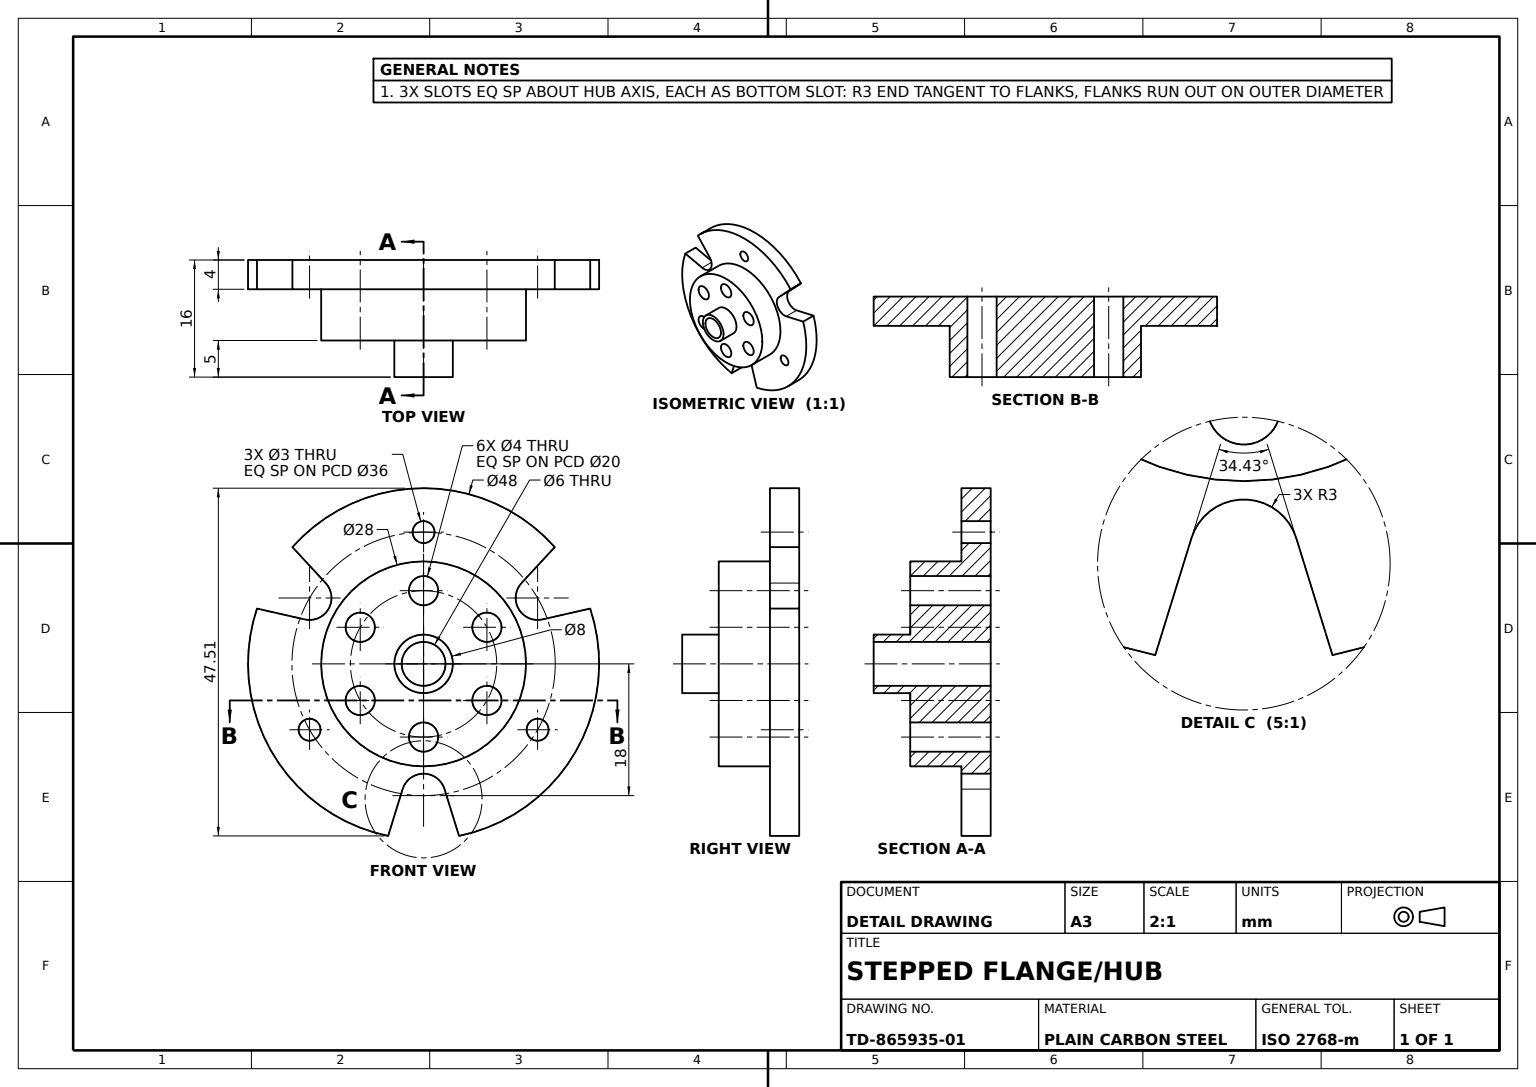
from build123d import *

# Parameters (mm, degrees)
SLOTTED_FLANGE_48_DEPTH = 4
HUB_SKETCH_R            = 14
HUB_28_DEPTH            = 7
HUB_HOLES_SKETCH_R      = 2
HUB_HOLES_6X_4_DEPTH    = 30
SPIGOT_SKETCH_R         = 4
SPIGOT_8_DEPTH          = 5
BORE_SKETCH_R           = 3
BORE_6_DEPTH            = 50
FLANGE_HOLES_SKETCH_R   = 1.5
FLANGE_HOLES_3X_3_DEPTH = 30


with BuildPart() as part:
    # Flange Profile Sketch → Slotted Flange Ø48 (new body)
    with BuildSketch(Plane.XY):
        with BuildLine():
            Line((4.846767643, -23.505506661), (2.865571245, -17.112023963))
            ThreePointArc((2.865571245, -17.112023963), (0, -15), (-2.865571245, -17.112023963))
            Line((-2.865571245, -17.112023963), (-4.846767643, -23.505506661))
            ThreePointArc((-4.846767643, -23.505506661), (-20.784609691, -12), (-22.779749719, 7.555329425))
            Line((-22.779749719, 7.555329425), (-16.252233084, 6.074354487))
            ThreePointArc((-16.252233084, 6.074354487), (-12.990381057, 7.5), (-13.38666184, 11.037669476))
            Line((-13.38666184, 11.037669476), (-17.932982076, 15.950177236))
            ThreePointArc((-17.932982076, 15.950177236), (0, 24), (17.932982076, 15.950177236))
            Line((17.932982076, 15.950177236), (13.38666184, 11.037669476))
            ThreePointArc((13.38666184, 11.037669476), (12.990381057, 7.5), (16.252233084, 6.074354487))
            Line((16.252233084, 6.074354487), (22.779749719, 7.555329425))
            ThreePointArc((22.779749719, 7.555329425), (20.784609691, -12), (4.846767643, -23.505506661))
        make_face()
    extrude(amount=SLOTTED_FLANGE_48_DEPTH)

    # Hub Sketch → Hub Ø28 (add)
    with BuildSketch(Plane.XY.offset(4)):
        Circle(HUB_SKETCH_R)
    extrude(amount=HUB_28_DEPTH)

    # Hub Holes Sketch → Hub Holes 6xØ4 (cut)
    with BuildSketch(Plane.XY.offset(11)):
        with Locations((0, 10)):
            Circle(HUB_HOLES_SKETCH_R)
        with Locations((8.660254038, 5)):
            Circle(HUB_HOLES_SKETCH_R)
        with Locations((8.660254038, -5)):
            Circle(HUB_HOLES_SKETCH_R)
        with Locations((0, -10)):
            Circle(HUB_HOLES_SKETCH_R)
        with Locations((-8.660254038, -5)):
            Circle(HUB_HOLES_SKETCH_R)
        with Locations((-8.660254038, 5)):
            Circle(HUB_HOLES_SKETCH_R)
    extrude(amount=-HUB_HOLES_6X_4_DEPTH, mode=Mode.SUBTRACT)

    # Spigot Sketch → Spigot Ø8 (add)
    with BuildSketch(Plane.XY.offset(11)):
        Circle(SPIGOT_SKETCH_R)
    extrude(amount=SPIGOT_8_DEPTH)

    # Bore Sketch → Bore Ø6 (cut)
    with BuildSketch(Plane.XY.offset(16)):
        Circle(BORE_SKETCH_R)
    extrude(amount=-BORE_6_DEPTH, mode=Mode.SUBTRACT)

    # Flange Holes Sketch → Flange Holes 3xØ3 (cut)
    with BuildSketch(Plane.XY.offset(4)):
        with Locations((15.588457268, -9)):
            Circle(FLANGE_HOLES_SKETCH_R)
        with Locations((0, 18)):
            Circle(FLANGE_HOLES_SKETCH_R)
        with Locations((-15.588457268, -9)):
            Circle(FLANGE_HOLES_SKETCH_R)
    extrude(amount=-FLANGE_HOLES_3X_3_DEPTH, mode=Mode.SUBTRACT)


solid = part.part
